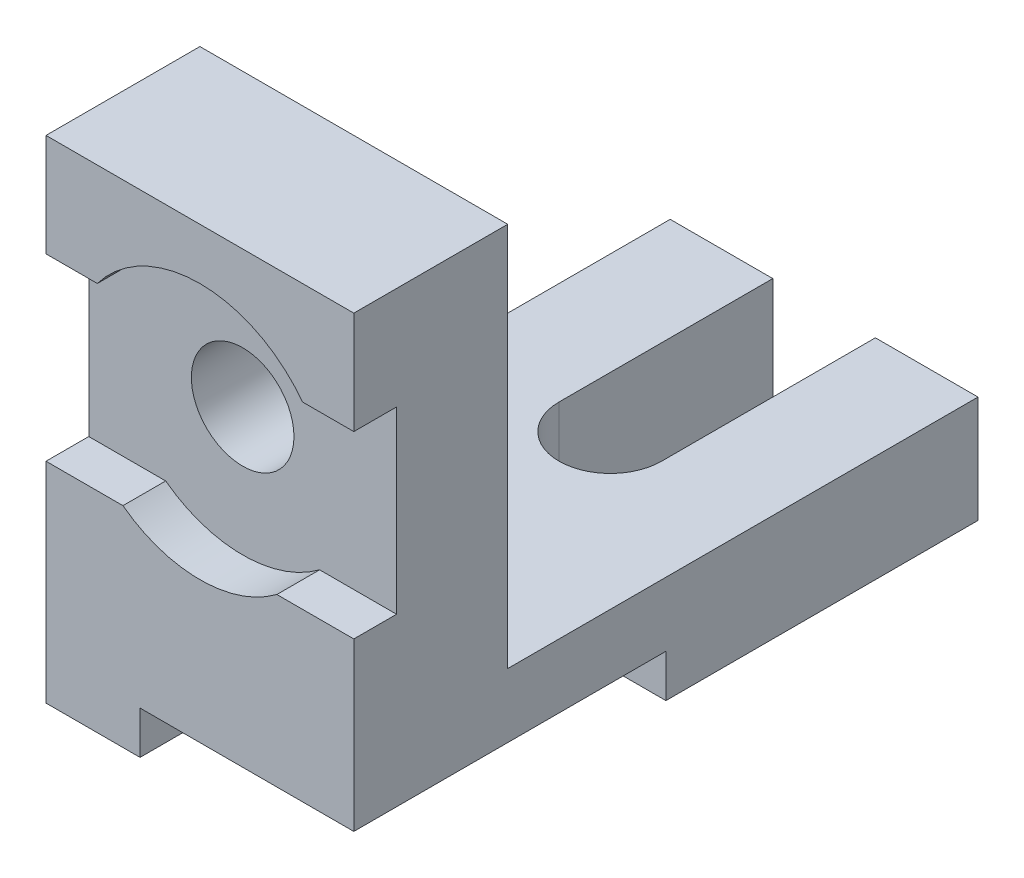
ISO-10303-21;
HEADER;
FILE_DESCRIPTION(('STEP AP214'),'2;1');
FILE_NAME('part.step','',(''),(''),'','','');
FILE_SCHEMA(('AUTOMOTIVE_DESIGN { 1 0 10303 214 1 1 1 1 }'));
ENDSEC;
DATA;
#1=APPLICATION_CONTEXT('core data for automotive mechanical design processes');
#2=APPLICATION_PROTOCOL_DEFINITION('international standard','automotive_design',2000,#1);
#3=PRODUCT_CONTEXT('',#1,'mechanical');
#4=PRODUCT('Part','Part','',(#3));
#5=PRODUCT_RELATED_PRODUCT_CATEGORY('part','',(#4));
#6=PRODUCT_DEFINITION_FORMATION('','',#4);
#7=PRODUCT_DEFINITION_CONTEXT('part definition',#1,'design');
#8=PRODUCT_DEFINITION('design','',#6,#7);
#9=PRODUCT_DEFINITION_SHAPE('','',#8);
#10=(LENGTH_UNIT() NAMED_UNIT(*) SI_UNIT(.MILLI.,.METRE.));
#11=(NAMED_UNIT(*) PLANE_ANGLE_UNIT() SI_UNIT($,.RADIAN.));
#12=(NAMED_UNIT(*) SI_UNIT($,.STERADIAN.) SOLID_ANGLE_UNIT());
#13=UNCERTAINTY_MEASURE_WITH_UNIT(LENGTH_MEASURE(1.E-05),#10,'distance_accuracy_value','');
#14=(GEOMETRIC_REPRESENTATION_CONTEXT(3) GLOBAL_UNCERTAINTY_ASSIGNED_CONTEXT((#13)) GLOBAL_UNIT_ASSIGNED_CONTEXT((#10,
#11,#12)) REPRESENTATION_CONTEXT('',''));
#15=CARTESIAN_POINT('',(0.,0.,0.));
#16=DIRECTION('',(0.,0.,1.));
#17=DIRECTION('',(1.,0.,0.));
#18=AXIS2_PLACEMENT_3D('',#15,#16,#17);
#19=CARTESIAN_POINT('',(-148.124947257375,-25.,-146.));
#20=DIRECTION('',(0.,0.,-1.));
#21=DIRECTION('',(-1.,0.,0.));
#22=AXIS2_PLACEMENT_3D('',#19,#20,#21);
#23=PLANE('',#22);
#24=DIRECTION('',(0.,1.,0.));
#25=VECTOR('',#24,1.);
#26=CARTESIAN_POINT('',(48.,-42.,-146.));
#27=LINE('',#26,#25);
#28=CARTESIAN_POINT('',(48.,-25.,-146.));
#29=VERTEX_POINT('',#28);
#30=CARTESIAN_POINT('',(48.,0.,-146.));
#31=VERTEX_POINT('',#30);
#32=EDGE_CURVE('E216',#29,#31,#27,.T.);
#33=ORIENTED_EDGE('',*,*,#32,.T.);
#34=DIRECTION('',(1.,0.,0.));
#35=VECTOR('',#34,1.);
#36=CARTESIAN_POINT('',(-148.124947257375,0.,-146.));
#37=LINE('',#36,#35);
#38=CARTESIAN_POINT('',(72.,0.,-146.));
#39=VERTEX_POINT('',#38);
#40=EDGE_CURVE('E247',#31,#39,#37,.T.);
#41=ORIENTED_EDGE('',*,*,#40,.T.);
#42=DIRECTION('',(0.,1.,0.));
#43=VECTOR('',#42,1.);
#44=CARTESIAN_POINT('',(72.,-25.,-146.));
#45=LINE('',#44,#43);
#46=CARTESIAN_POINT('',(72.,-25.,-146.));
#47=VERTEX_POINT('',#46);
#48=EDGE_CURVE('E231',#47,#39,#45,.T.);
#49=ORIENTED_EDGE('',*,*,#48,.F.);
#50=DIRECTION('',(1.,0.,0.));
#51=VECTOR('',#50,1.);
#52=CARTESIAN_POINT('',(-148.124947257375,-25.,-146.));
#53=LINE('',#52,#51);
#54=EDGE_CURVE('E252',#29,#47,#53,.T.);
#55=ORIENTED_EDGE('',*,*,#54,.F.);
#56=EDGE_LOOP('',(#33,#41,#49,#55));
#57=FACE_BOUND('',#56,.T.);
#58=ADVANCED_FACE('F39',(#57),#23,.T.);
#59=CARTESIAN_POINT('',(0.,0.,0.));
#60=DIRECTION('',(0.,0.,-1.));
#61=DIRECTION('',(-1.,0.,0.));
#62=AXIS2_PLACEMENT_3D('',#59,#60,#61);
#63=PLANE('',#62);
#64=DIRECTION('',(0.,-1.,0.));
#65=VECTOR('',#64,1.);
#66=CARTESIAN_POINT('',(0.,0.,0.));
#67=LINE('',#66,#65);
#68=CARTESIAN_POINT('',(0.,90.,0.));
#69=VERTEX_POINT('',#68);
#70=CARTESIAN_POINT('',(0.,66.,0.));
#71=VERTEX_POINT('',#70);
#72=EDGE_CURVE('E333',#69,#71,#67,.T.);
#73=ORIENTED_EDGE('',*,*,#72,.T.);
#74=DIRECTION('',(-1.,0.,0.));
#75=VECTOR('',#74,1.);
#76=CARTESIAN_POINT('',(0.,66.,0.));
#77=LINE('',#76,#75);
#78=CARTESIAN_POINT('',(12.,66.,0.));
#79=VERTEX_POINT('',#78);
#80=EDGE_CURVE('E297',#79,#71,#77,.T.);
#81=ORIENTED_EDGE('',*,*,#80,.F.);
#82=CARTESIAN_POINT('',(36.,48.,0.));
#83=DIRECTION('',(0.,0.,1.));
#84=DIRECTION('',(1.,0.,0.));
#85=AXIS2_PLACEMENT_3D('',#82,#83,#84);
#86=CIRCLE('',#85,30.);
#87=CARTESIAN_POINT('',(60.,66.,0.));
#88=VERTEX_POINT('',#87);
#89=EDGE_CURVE('E300',#88,#79,#86,.T.);
#90=ORIENTED_EDGE('',*,*,#89,.F.);
#91=DIRECTION('',(-1.,0.,0.));
#92=VECTOR('',#91,1.);
#93=CARTESIAN_POINT('',(60.,66.,0.));
#94=LINE('',#93,#92);
#95=CARTESIAN_POINT('',(72.,66.,0.));
#96=VERTEX_POINT('',#95);
#97=EDGE_CURVE('E294',#96,#88,#94,.T.);
#98=ORIENTED_EDGE('',*,*,#97,.F.);
#99=DIRECTION('',(0.,1.,0.));
#100=VECTOR('',#99,1.);
#101=CARTESIAN_POINT('',(72.,0.,0.));
#102=LINE('',#101,#100);
#103=CARTESIAN_POINT('',(72.,90.,0.));
#104=VERTEX_POINT('',#103);
#105=EDGE_CURVE('E336',#96,#104,#102,.T.);
#106=ORIENTED_EDGE('',*,*,#105,.T.);
#107=DIRECTION('',(-1.,0.,0.));
#108=VECTOR('',#107,1.);
#109=CARTESIAN_POINT('',(0.,90.,0.));
#110=LINE('',#109,#108);
#111=EDGE_CURVE('E326',#104,#69,#110,.T.);
#112=ORIENTED_EDGE('',*,*,#111,.T.);
#113=EDGE_LOOP('',(#73,#81,#90,#98,#106,#112));
#114=FACE_BOUND('',#113,.T.);
#115=ADVANCED_FACE('F344',(#114),#63,.F.);
#116=CARTESIAN_POINT('',(0.,0.,-36.));
#117=DIRECTION('',(-1.,0.,0.));
#118=DIRECTION('',(0.,0.,1.));
#119=AXIS2_PLACEMENT_3D('',#116,#117,#118);
#120=PLANE('',#119);
#121=DIRECTION('',(0.,0.,1.));
#122=VECTOR('',#121,1.);
#123=CARTESIAN_POINT('',(0.,24.,-10.));
#124=LINE('',#123,#122);
#125=CARTESIAN_POINT('',(0.,24.,-10.));
#126=VERTEX_POINT('',#125);
#127=CARTESIAN_POINT('',(0.,24.,0.));
#128=VERTEX_POINT('',#127);
#129=EDGE_CURVE('E307',#126,#128,#124,.T.);
#130=ORIENTED_EDGE('',*,*,#129,.F.);
#131=DIRECTION('',(0.,-1.,0.));
#132=VECTOR('',#131,1.);
#133=CARTESIAN_POINT('',(0.,66.,-10.));
#134=LINE('',#133,#132);
#135=CARTESIAN_POINT('',(0.,66.,-10.));
#136=VERTEX_POINT('',#135);
#137=EDGE_CURVE('E284',#136,#126,#134,.T.);
#138=ORIENTED_EDGE('',*,*,#137,.F.);
#139=DIRECTION('',(0.,0.,1.));
#140=VECTOR('',#139,1.);
#141=CARTESIAN_POINT('',(0.,66.,-10.));
#142=LINE('',#141,#140);
#143=EDGE_CURVE('E310',#136,#71,#142,.T.);
#144=ORIENTED_EDGE('',*,*,#143,.T.);
#145=ORIENTED_EDGE('',*,*,#72,.F.);
#146=DIRECTION('',(0.,0.,1.));
#147=VECTOR('',#146,1.);
#148=CARTESIAN_POINT('',(0.,90.,-36.));
#149=LINE('',#148,#147);
#150=CARTESIAN_POINT('',(0.,90.,-36.));
#151=VERTEX_POINT('',#150);
#152=EDGE_CURVE('E11',#151,#69,#149,.T.);
#153=ORIENTED_EDGE('',*,*,#152,.F.);
#154=DIRECTION('',(0.,-1.,0.));
#155=VECTOR('',#154,1.);
#156=CARTESIAN_POINT('',(0.,0.,-36.));
#157=LINE('',#156,#155);
#158=CARTESIAN_POINT('',(0.,0.,-36.));
#159=VERTEX_POINT('',#158);
#160=EDGE_CURVE('E325',#151,#159,#157,.T.);
#161=ORIENTED_EDGE('',*,*,#160,.T.);
#162=DIRECTION('',(0.,0.,1.));
#163=VECTOR('',#162,1.);
#164=CARTESIAN_POINT('',(0.,0.,-146.));
#165=LINE('',#164,#163);
#166=CARTESIAN_POINT('',(0.,0.,-146.));
#167=VERTEX_POINT('',#166);
#168=EDGE_CURVE('E239',#167,#159,#165,.T.);
#169=ORIENTED_EDGE('',*,*,#168,.F.);
#170=DIRECTION('',(0.,1.,0.));
#171=VECTOR('',#170,1.);
#172=CARTESIAN_POINT('',(0.,-25.,-146.));
#173=LINE('',#172,#171);
#174=CARTESIAN_POINT('',(0.,-25.,-146.));
#175=VERTEX_POINT('',#174);
#176=EDGE_CURVE('E244',#175,#167,#173,.T.);
#177=ORIENTED_EDGE('',*,*,#176,.F.);
#178=DIRECTION('',(0.,0.,-1.));
#179=VECTOR('',#178,1.);
#180=CARTESIAN_POINT('',(0.,-25.,0.));
#181=LINE('',#180,#179);
#182=CARTESIAN_POINT('',(0.,-25.,0.));
#183=VERTEX_POINT('',#182);
#184=EDGE_CURVE('E248',#183,#175,#181,.T.);
#185=ORIENTED_EDGE('',*,*,#184,.F.);
#186=EDGE_CURVE('E308',#128,#183,#67,.T.);
#187=ORIENTED_EDGE('',*,*,#186,.F.);
#188=EDGE_LOOP('',(#130,#138,#144,#145,#153,#161,#169,#177,#185,#187));
#189=FACE_BOUND('',#188,.T.);
#190=ADVANCED_FACE('F41',(#189),#120,.T.);
#191=CARTESIAN_POINT('',(0.,90.,-36.));
#192=DIRECTION('',(0.,1.,0.));
#193=DIRECTION('',(0.,0.,1.));
#194=AXIS2_PLACEMENT_3D('',#191,#192,#193);
#195=PLANE('',#194);
#196=ORIENTED_EDGE('',*,*,#111,.F.);
#197=DIRECTION('',(0.,0.,1.));
#198=VECTOR('',#197,1.);
#199=CARTESIAN_POINT('',(72.,90.,-36.));
#200=LINE('',#199,#198);
#201=CARTESIAN_POINT('',(72.,90.,-36.));
#202=VERTEX_POINT('',#201);
#203=EDGE_CURVE('E43',#202,#104,#200,.T.);
#204=ORIENTED_EDGE('',*,*,#203,.F.);
#205=DIRECTION('',(-1.,0.,0.));
#206=VECTOR('',#205,1.);
#207=CARTESIAN_POINT('',(0.,90.,-36.));
#208=LINE('',#207,#206);
#209=EDGE_CURVE('E335',#202,#151,#208,.T.);
#210=ORIENTED_EDGE('',*,*,#209,.T.);
#211=ORIENTED_EDGE('',*,*,#152,.T.);
#212=EDGE_LOOP('',(#196,#204,#210,#211));
#213=FACE_BOUND('',#212,.T.);
#214=ADVANCED_FACE('F348',(#213),#195,.T.);
#215=CARTESIAN_POINT('',(72.,0.,-36.));
#216=DIRECTION('',(1.,0.,0.));
#217=DIRECTION('',(0.,0.,-1.));
#218=AXIS2_PLACEMENT_3D('',#215,#216,#217);
#219=PLANE('',#218);
#220=DIRECTION('',(0.,0.,1.));
#221=VECTOR('',#220,1.);
#222=CARTESIAN_POINT('',(72.,-15.,-73.));
#223=LINE('',#222,#221);
#224=CARTESIAN_POINT('',(72.,-15.,-73.));
#225=VERTEX_POINT('',#224);
#226=CARTESIAN_POINT('',(72.,-15.,0.));
#227=VERTEX_POINT('',#226);
#228=EDGE_CURVE('E188',#225,#227,#223,.T.);
#229=ORIENTED_EDGE('',*,*,#228,.F.);
#230=DIRECTION('',(0.,1.,0.));
#231=VECTOR('',#230,1.);
#232=CARTESIAN_POINT('',(72.,-25.,-73.));
#233=LINE('',#232,#231);
#234=CARTESIAN_POINT('',(72.,-25.,-73.));
#235=VERTEX_POINT('',#234);
#236=EDGE_CURVE('E189',#235,#225,#233,.T.);
#237=ORIENTED_EDGE('',*,*,#236,.F.);
#238=DIRECTION('',(0.,0.,-1.));
#239=VECTOR('',#238,1.);
#240=CARTESIAN_POINT('',(72.,-25.,0.));
#241=LINE('',#240,#239);
#242=EDGE_CURVE('E235',#235,#47,#241,.T.);
#243=ORIENTED_EDGE('',*,*,#242,.T.);
#244=ORIENTED_EDGE('',*,*,#48,.T.);
#245=DIRECTION('',(0.,0.,1.));
#246=VECTOR('',#245,1.);
#247=CARTESIAN_POINT('',(72.,0.,-146.));
#248=LINE('',#247,#246);
#249=CARTESIAN_POINT('',(72.,0.,-36.));
#250=VERTEX_POINT('',#249);
#251=EDGE_CURVE('E227',#39,#250,#248,.T.);
#252=ORIENTED_EDGE('',*,*,#251,.T.);
#253=DIRECTION('',(0.,1.,0.));
#254=VECTOR('',#253,1.);
#255=CARTESIAN_POINT('',(72.,0.,-36.));
#256=LINE('',#255,#254);
#257=EDGE_CURVE('E328',#250,#202,#256,.T.);
#258=ORIENTED_EDGE('',*,*,#257,.T.);
#259=ORIENTED_EDGE('',*,*,#203,.T.);
#260=ORIENTED_EDGE('',*,*,#105,.F.);
#261=DIRECTION('',(0.,0.,1.));
#262=VECTOR('',#261,1.);
#263=CARTESIAN_POINT('',(72.,66.,-10.));
#264=LINE('',#263,#262);
#265=CARTESIAN_POINT('',(72.,66.,-10.));
#266=VERTEX_POINT('',#265);
#267=EDGE_CURVE('E316',#266,#96,#264,.T.);
#268=ORIENTED_EDGE('',*,*,#267,.F.);
#269=DIRECTION('',(0.,1.,0.));
#270=VECTOR('',#269,1.);
#271=CARTESIAN_POINT('',(72.,24.,-10.));
#272=LINE('',#271,#270);
#273=CARTESIAN_POINT('',(72.,24.,-10.));
#274=VERTEX_POINT('',#273);
#275=EDGE_CURVE('E275',#274,#266,#272,.T.);
#276=ORIENTED_EDGE('',*,*,#275,.F.);
#277=DIRECTION('',(0.,0.,1.));
#278=VECTOR('',#277,1.);
#279=CARTESIAN_POINT('',(72.,24.,-10.));
#280=LINE('',#279,#278);
#281=CARTESIAN_POINT('',(72.,24.,0.));
#282=VERTEX_POINT('',#281);
#283=EDGE_CURVE('E318',#274,#282,#280,.T.);
#284=ORIENTED_EDGE('',*,*,#283,.T.);
#285=EDGE_CURVE('E205',#227,#282,#102,.T.);
#286=ORIENTED_EDGE('',*,*,#285,.F.);
#287=EDGE_LOOP('',(#229,#237,#243,#244,#252,#258,#259,#260,#268,#276,#284,#286));
#288=FACE_BOUND('',#287,.T.);
#289=ADVANCED_FACE('F199',(#288),#219,.T.);
#290=CARTESIAN_POINT('',(0.,0.,-36.));
#291=DIRECTION('',(0.,0.,-1.));
#292=DIRECTION('',(-1.,0.,0.));
#293=AXIS2_PLACEMENT_3D('',#290,#291,#292);
#294=PLANE('',#293);
#295=CARTESIAN_POINT('',(36.,48.,-36.));
#296=DIRECTION('',(0.,0.,-1.));
#297=DIRECTION('',(-1.,0.,0.));
#298=AXIS2_PLACEMENT_3D('',#295,#296,#297);
#299=CIRCLE('',#298,12.);
#300=CARTESIAN_POINT('',(24.,48.,-36.));
#301=VERTEX_POINT('',#300);
#302=EDGE_CURVE('E261',#301,#301,#299,.T.);
#303=ORIENTED_EDGE('',*,*,#302,.F.);
#304=EDGE_LOOP('',(#303));
#305=FACE_BOUND('',#304,.T.);
#306=ORIENTED_EDGE('',*,*,#160,.F.);
#307=ORIENTED_EDGE('',*,*,#209,.F.);
#308=ORIENTED_EDGE('',*,*,#257,.F.);
#309=DIRECTION('',(1.,0.,0.));
#310=VECTOR('',#309,1.);
#311=CARTESIAN_POINT('',(0.,0.,-36.));
#312=LINE('',#311,#310);
#313=EDGE_CURVE('E324',#159,#250,#312,.T.);
#314=ORIENTED_EDGE('',*,*,#313,.F.);
#315=EDGE_LOOP('',(#306,#307,#308,#314));
#316=FACE_BOUND('',#315,.T.);
#317=ADVANCED_FACE('F371',(#305,#316),#294,.T.);
#318=DIRECTION('',(1.,0.,0.));
#319=VECTOR('',#318,1.);
#320=CARTESIAN_POINT('',(-148.124947257375,-25.,0.));
#321=LINE('',#320,#319);
#322=CARTESIAN_POINT('',(22.,-25.,0.));
#323=VERTEX_POINT('',#322);
#324=EDGE_CURVE('E233',#183,#323,#321,.T.);
#325=ORIENTED_EDGE('',*,*,#324,.T.);
#326=DIRECTION('',(0.,-1.,0.));
#327=VECTOR('',#326,1.);
#328=CARTESIAN_POINT('',(22.,-25.,0.));
#329=LINE('',#328,#327);
#330=CARTESIAN_POINT('',(22.,-15.,0.));
#331=VERTEX_POINT('',#330);
#332=EDGE_CURVE('E197',#331,#323,#329,.T.);
#333=ORIENTED_EDGE('',*,*,#332,.F.);
#334=DIRECTION('',(-1.,0.,0.));
#335=VECTOR('',#334,1.);
#336=CARTESIAN_POINT('',(72.,-15.,0.));
#337=LINE('',#336,#335);
#338=EDGE_CURVE('E400',#227,#331,#337,.T.);
#339=ORIENTED_EDGE('',*,*,#338,.F.);
#340=ORIENTED_EDGE('',*,*,#285,.T.);
#341=DIRECTION('',(1.,0.,0.));
#342=VECTOR('',#341,1.);
#343=CARTESIAN_POINT('',(54.,24.,0.));
#344=LINE('',#343,#342);
#345=CARTESIAN_POINT('',(54.,24.,0.));
#346=VERTEX_POINT('',#345);
#347=EDGE_CURVE('E292',#346,#282,#344,.T.);
#348=ORIENTED_EDGE('',*,*,#347,.F.);
#349=CARTESIAN_POINT('',(36.,48.,0.));
#350=DIRECTION('',(0.,0.,1.));
#351=DIRECTION('',(1.,0.,0.));
#352=AXIS2_PLACEMENT_3D('',#349,#350,#351);
#353=CIRCLE('',#352,30.);
#354=CARTESIAN_POINT('',(18.,24.,0.));
#355=VERTEX_POINT('',#354);
#356=EDGE_CURVE('E262',#355,#346,#353,.T.);
#357=ORIENTED_EDGE('',*,*,#356,.F.);
#358=DIRECTION('',(1.,0.,0.));
#359=VECTOR('',#358,1.);
#360=CARTESIAN_POINT('',(0.,24.,0.));
#361=LINE('',#360,#359);
#362=EDGE_CURVE('E267',#128,#355,#361,.T.);
#363=ORIENTED_EDGE('',*,*,#362,.F.);
#364=ORIENTED_EDGE('',*,*,#186,.T.);
#365=EDGE_LOOP('',(#325,#333,#339,#340,#348,#357,#363,#364));
#366=FACE_BOUND('',#365,.T.);
#367=ADVANCED_FACE('F389',(#366),#63,.F.);
#368=CARTESIAN_POINT('',(36.,48.,-10.));
#369=DIRECTION('',(0.,0.,1.));
#370=DIRECTION('',(1.,0.,0.));
#371=AXIS2_PLACEMENT_3D('',#368,#369,#370);
#372=CYLINDRICAL_SURFACE('',#371,30.);
#373=ORIENTED_EDGE('',*,*,#356,.T.);
#374=DIRECTION('',(0.,0.,1.));
#375=VECTOR('',#374,1.);
#376=CARTESIAN_POINT('',(54.,24.,-10.));
#377=LINE('',#376,#375);
#378=CARTESIAN_POINT('',(54.,24.,-10.));
#379=VERTEX_POINT('',#378);
#380=EDGE_CURVE('E288',#379,#346,#377,.T.);
#381=ORIENTED_EDGE('',*,*,#380,.F.);
#382=CARTESIAN_POINT('',(36.,48.,-10.));
#383=DIRECTION('',(0.,0.,1.));
#384=DIRECTION('',(1.,0.,0.));
#385=AXIS2_PLACEMENT_3D('',#382,#383,#384);
#386=CIRCLE('',#385,30.);
#387=CARTESIAN_POINT('',(18.,24.,-10.));
#388=VERTEX_POINT('',#387);
#389=EDGE_CURVE('E264',#388,#379,#386,.T.);
#390=ORIENTED_EDGE('',*,*,#389,.F.);
#391=DIRECTION('',(0.,0.,1.));
#392=VECTOR('',#391,1.);
#393=CARTESIAN_POINT('',(18.,24.,-10.));
#394=LINE('',#393,#392);
#395=EDGE_CURVE('E303',#388,#355,#394,.T.);
#396=ORIENTED_EDGE('',*,*,#395,.T.);
#397=EDGE_LOOP('',(#373,#381,#390,#396));
#398=FACE_BOUND('',#397,.T.);
#399=ADVANCED_FACE('F397',(#398),#372,.F.);
#400=CARTESIAN_POINT('',(0.,24.,-10.));
#401=DIRECTION('',(0.,-1.,0.));
#402=DIRECTION('',(0.,0.,-1.));
#403=AXIS2_PLACEMENT_3D('',#400,#401,#402);
#404=PLANE('',#403);
#405=ORIENTED_EDGE('',*,*,#362,.T.);
#406=ORIENTED_EDGE('',*,*,#395,.F.);
#407=DIRECTION('',(1.,0.,0.));
#408=VECTOR('',#407,1.);
#409=CARTESIAN_POINT('',(0.,24.,-10.));
#410=LINE('',#409,#408);
#411=EDGE_CURVE('E286',#126,#388,#410,.T.);
#412=ORIENTED_EDGE('',*,*,#411,.F.);
#413=ORIENTED_EDGE('',*,*,#129,.T.);
#414=EDGE_LOOP('',(#405,#406,#412,#413));
#415=FACE_BOUND('',#414,.T.);
#416=ADVANCED_FACE('F391',(#415),#404,.F.);
#417=CARTESIAN_POINT('',(0.,66.,-10.));
#418=DIRECTION('',(0.,1.,0.));
#419=DIRECTION('',(0.,0.,1.));
#420=AXIS2_PLACEMENT_3D('',#417,#418,#419);
#421=PLANE('',#420);
#422=ORIENTED_EDGE('',*,*,#80,.T.);
#423=ORIENTED_EDGE('',*,*,#143,.F.);
#424=DIRECTION('',(-1.,0.,0.));
#425=VECTOR('',#424,1.);
#426=CARTESIAN_POINT('',(0.,66.,-10.));
#427=LINE('',#426,#425);
#428=CARTESIAN_POINT('',(12.,66.,-10.));
#429=VERTEX_POINT('',#428);
#430=EDGE_CURVE('E283',#429,#136,#427,.T.);
#431=ORIENTED_EDGE('',*,*,#430,.F.);
#432=DIRECTION('',(0.,0.,1.));
#433=VECTOR('',#432,1.);
#434=CARTESIAN_POINT('',(12.,66.,-10.));
#435=LINE('',#434,#433);
#436=EDGE_CURVE('E315',#429,#79,#435,.T.);
#437=ORIENTED_EDGE('',*,*,#436,.T.);
#438=EDGE_LOOP('',(#422,#423,#431,#437));
#439=FACE_BOUND('',#438,.T.);
#440=ADVANCED_FACE('F359',(#439),#421,.F.);
#441=CARTESIAN_POINT('',(36.,48.,-10.));
#442=DIRECTION('',(0.,0.,1.));
#443=DIRECTION('',(1.,0.,0.));
#444=AXIS2_PLACEMENT_3D('',#441,#442,#443);
#445=CYLINDRICAL_SURFACE('',#444,30.);
#446=ORIENTED_EDGE('',*,*,#89,.T.);
#447=ORIENTED_EDGE('',*,*,#436,.F.);
#448=CARTESIAN_POINT('',(36.,48.,-10.));
#449=DIRECTION('',(0.,0.,1.));
#450=DIRECTION('',(1.,0.,0.));
#451=AXIS2_PLACEMENT_3D('',#448,#449,#450);
#452=CIRCLE('',#451,30.);
#453=CARTESIAN_POINT('',(60.,66.,-10.));
#454=VERTEX_POINT('',#453);
#455=EDGE_CURVE('E279',#454,#429,#452,.T.);
#456=ORIENTED_EDGE('',*,*,#455,.F.);
#457=DIRECTION('',(0.,0.,1.));
#458=VECTOR('',#457,1.);
#459=CARTESIAN_POINT('',(60.,66.,-10.));
#460=LINE('',#459,#458);
#461=EDGE_CURVE('E314',#454,#88,#460,.T.);
#462=ORIENTED_EDGE('',*,*,#461,.T.);
#463=EDGE_LOOP('',(#446,#447,#456,#462));
#464=FACE_BOUND('',#463,.T.);
#465=ADVANCED_FACE('F365',(#464),#445,.F.);
#466=CARTESIAN_POINT('',(60.,66.,-10.));
#467=DIRECTION('',(0.,1.,0.));
#468=DIRECTION('',(0.,0.,1.));
#469=AXIS2_PLACEMENT_3D('',#466,#467,#468);
#470=PLANE('',#469);
#471=ORIENTED_EDGE('',*,*,#97,.T.);
#472=ORIENTED_EDGE('',*,*,#461,.F.);
#473=DIRECTION('',(-1.,0.,0.));
#474=VECTOR('',#473,1.);
#475=CARTESIAN_POINT('',(60.,66.,-10.));
#476=LINE('',#475,#474);
#477=EDGE_CURVE('E274',#266,#454,#476,.T.);
#478=ORIENTED_EDGE('',*,*,#477,.F.);
#479=ORIENTED_EDGE('',*,*,#267,.T.);
#480=EDGE_LOOP('',(#471,#472,#478,#479));
#481=FACE_BOUND('',#480,.T.);
#482=ADVANCED_FACE('F463',(#481),#470,.F.);
#483=CARTESIAN_POINT('',(54.,24.,-10.));
#484=DIRECTION('',(0.,-1.,0.));
#485=DIRECTION('',(0.,0.,-1.));
#486=AXIS2_PLACEMENT_3D('',#483,#484,#485);
#487=PLANE('',#486);
#488=ORIENTED_EDGE('',*,*,#347,.T.);
#489=ORIENTED_EDGE('',*,*,#283,.F.);
#490=DIRECTION('',(1.,0.,0.));
#491=VECTOR('',#490,1.);
#492=CARTESIAN_POINT('',(54.,24.,-10.));
#493=LINE('',#492,#491);
#494=EDGE_CURVE('E268',#379,#274,#493,.T.);
#495=ORIENTED_EDGE('',*,*,#494,.F.);
#496=ORIENTED_EDGE('',*,*,#380,.T.);
#497=EDGE_LOOP('',(#488,#489,#495,#496));
#498=FACE_BOUND('',#497,.T.);
#499=ADVANCED_FACE('F398',(#498),#487,.F.);
#500=CARTESIAN_POINT('',(36.,48.,-10.));
#501=DIRECTION('',(0.,0.,1.));
#502=DIRECTION('',(1.,0.,0.));
#503=AXIS2_PLACEMENT_3D('',#500,#501,#502);
#504=PLANE('',#503);
#505=CARTESIAN_POINT('',(36.,48.,-10.));
#506=DIRECTION('',(0.,0.,1.));
#507=DIRECTION('',(1.,0.,0.));
#508=AXIS2_PLACEMENT_3D('',#505,#506,#507);
#509=CIRCLE('',#508,12.);
#510=CARTESIAN_POINT('',(48.,48.,-10.));
#511=VERTEX_POINT('',#510);
#512=EDGE_CURVE('E245',#511,#511,#509,.T.);
#513=ORIENTED_EDGE('',*,*,#512,.F.);
#514=EDGE_LOOP('',(#513));
#515=FACE_BOUND('',#514,.T.);
#516=ORIENTED_EDGE('',*,*,#389,.T.);
#517=ORIENTED_EDGE('',*,*,#494,.T.);
#518=ORIENTED_EDGE('',*,*,#275,.T.);
#519=ORIENTED_EDGE('',*,*,#477,.T.);
#520=ORIENTED_EDGE('',*,*,#455,.T.);
#521=ORIENTED_EDGE('',*,*,#430,.T.);
#522=ORIENTED_EDGE('',*,*,#137,.T.);
#523=ORIENTED_EDGE('',*,*,#411,.T.);
#524=EDGE_LOOP('',(#516,#517,#518,#519,#520,#521,#522,#523));
#525=FACE_BOUND('',#524,.T.);
#526=ADVANCED_FACE('F360',(#515,#525),#504,.T.);
#527=CARTESIAN_POINT('',(36.,48.,-52.));
#528=DIRECTION('',(0.,0.,1.));
#529=DIRECTION('',(1.,0.,0.));
#530=AXIS2_PLACEMENT_3D('',#527,#528,#529);
#531=CYLINDRICAL_SURFACE('',#530,12.);
#532=ORIENTED_EDGE('',*,*,#302,.T.);
#533=EDGE_LOOP('',(#532));
#534=FACE_BOUND('',#533,.T.);
#535=ORIENTED_EDGE('',*,*,#512,.T.);
#536=EDGE_LOOP('',(#535));
#537=FACE_BOUND('',#536,.T.);
#538=ADVANCED_FACE('F441',(#534,#537),#531,.F.);
#539=CARTESIAN_POINT('',(-148.124947257375,-25.,0.));
#540=DIRECTION('',(0.,-1.,0.));
#541=DIRECTION('',(0.,0.,-1.));
#542=AXIS2_PLACEMENT_3D('',#539,#540,#541);
#543=PLANE('',#542);
#544=DIRECTION('',(0.,0.,1.));
#545=VECTOR('',#544,1.);
#546=CARTESIAN_POINT('',(22.,-25.,-73.));
#547=LINE('',#546,#545);
#548=CARTESIAN_POINT('',(22.,-25.,-73.));
#549=VERTEX_POINT('',#548);
#550=EDGE_CURVE('E204',#549,#323,#547,.T.);
#551=ORIENTED_EDGE('',*,*,#550,.T.);
#552=ORIENTED_EDGE('',*,*,#324,.F.);
#553=ORIENTED_EDGE('',*,*,#184,.T.);
#554=CARTESIAN_POINT('',(24.,-25.,-146.));
#555=VERTEX_POINT('',#554);
#556=EDGE_CURVE('E249',#175,#555,#53,.T.);
#557=ORIENTED_EDGE('',*,*,#556,.T.);
#558=DIRECTION('',(0.,0.,-1.));
#559=VECTOR('',#558,1.);
#560=CARTESIAN_POINT('',(24.,-25.,0.));
#561=LINE('',#560,#559);
#562=CARTESIAN_POINT('',(24.,-25.,-96.));
#563=VERTEX_POINT('',#562);
#564=EDGE_CURVE('E218',#563,#555,#561,.T.);
#565=ORIENTED_EDGE('',*,*,#564,.F.);
#566=CARTESIAN_POINT('',(36.,-25.,-96.));
#567=DIRECTION('',(0.,-1.,0.));
#568=DIRECTION('',(0.,0.,-1.));
#569=AXIS2_PLACEMENT_3D('',#566,#567,#568);
#570=CIRCLE('',#569,12.);
#571=CARTESIAN_POINT('',(48.,-25.,-96.));
#572=VERTEX_POINT('',#571);
#573=EDGE_CURVE('E228',#572,#563,#570,.T.);
#574=ORIENTED_EDGE('',*,*,#573,.F.);
#575=DIRECTION('',(0.,0.,1.));
#576=VECTOR('',#575,1.);
#577=CARTESIAN_POINT('',(48.,-25.,0.));
#578=LINE('',#577,#576);
#579=EDGE_CURVE('E226',#29,#572,#578,.T.);
#580=ORIENTED_EDGE('',*,*,#579,.F.);
#581=ORIENTED_EDGE('',*,*,#54,.T.);
#582=ORIENTED_EDGE('',*,*,#242,.F.);
#583=DIRECTION('',(1.,0.,0.));
#584=VECTOR('',#583,1.);
#585=CARTESIAN_POINT('',(72.,-25.,-73.));
#586=LINE('',#585,#584);
#587=EDGE_CURVE('E193',#549,#235,#586,.T.);
#588=ORIENTED_EDGE('',*,*,#587,.F.);
#589=EDGE_LOOP('',(#551,#552,#553,#557,#565,#574,#580,#581,#582,#588));
#590=FACE_BOUND('',#589,.T.);
#591=ADVANCED_FACE('F384',(#590),#543,.T.);
#592=DIRECTION('',(0.,1.,0.));
#593=VECTOR('',#592,1.);
#594=CARTESIAN_POINT('',(24.,-42.,-146.));
#595=LINE('',#594,#593);
#596=CARTESIAN_POINT('',(24.,0.,-146.));
#597=VERTEX_POINT('',#596);
#598=EDGE_CURVE('E65',#555,#597,#595,.T.);
#599=ORIENTED_EDGE('',*,*,#598,.F.);
#600=ORIENTED_EDGE('',*,*,#556,.F.);
#601=ORIENTED_EDGE('',*,*,#176,.T.);
#602=EDGE_CURVE('E241',#167,#597,#37,.T.);
#603=ORIENTED_EDGE('',*,*,#602,.T.);
#604=EDGE_LOOP('',(#599,#600,#601,#603));
#605=FACE_BOUND('',#604,.T.);
#606=ADVANCED_FACE('F377',(#605),#23,.T.);
#607=CARTESIAN_POINT('',(-148.124947257375,0.,-146.));
#608=DIRECTION('',(0.,1.,0.));
#609=DIRECTION('',(0.,0.,1.));
#610=AXIS2_PLACEMENT_3D('',#607,#608,#609);
#611=PLANE('',#610);
#612=DIRECTION('',(0.,0.,-1.));
#613=VECTOR('',#612,1.);
#614=CARTESIAN_POINT('',(48.,0.,-96.));
#615=LINE('',#614,#613);
#616=CARTESIAN_POINT('',(48.,0.,-96.));
#617=VERTEX_POINT('',#616);
#618=EDGE_CURVE('E212',#617,#31,#615,.T.);
#619=ORIENTED_EDGE('',*,*,#618,.F.);
#620=CARTESIAN_POINT('',(36.,0.,-96.));
#621=DIRECTION('',(0.,1.,0.));
#622=DIRECTION('',(0.,0.,1.));
#623=AXIS2_PLACEMENT_3D('',#620,#621,#622);
#624=CIRCLE('',#623,12.);
#625=CARTESIAN_POINT('',(24.,0.,-96.));
#626=VERTEX_POINT('',#625);
#627=EDGE_CURVE('E211',#626,#617,#624,.T.);
#628=ORIENTED_EDGE('',*,*,#627,.F.);
#629=DIRECTION('',(0.,0.,1.));
#630=VECTOR('',#629,1.);
#631=CARTESIAN_POINT('',(24.,0.,-146.));
#632=LINE('',#631,#630);
#633=EDGE_CURVE('E207',#597,#626,#632,.T.);
#634=ORIENTED_EDGE('',*,*,#633,.F.);
#635=ORIENTED_EDGE('',*,*,#602,.F.);
#636=ORIENTED_EDGE('',*,*,#168,.T.);
#637=ORIENTED_EDGE('',*,*,#313,.T.);
#638=ORIENTED_EDGE('',*,*,#251,.F.);
#639=ORIENTED_EDGE('',*,*,#40,.F.);
#640=EDGE_LOOP('',(#619,#628,#634,#635,#636,#637,#638,#639));
#641=FACE_BOUND('',#640,.T.);
#642=ADVANCED_FACE('F374',(#641),#611,.T.);
#643=CARTESIAN_POINT('',(48.,-42.,-96.));
#644=DIRECTION('',(1.,0.,0.));
#645=DIRECTION('',(0.,0.,-1.));
#646=AXIS2_PLACEMENT_3D('',#643,#644,#645);
#647=PLANE('',#646);
#648=ORIENTED_EDGE('',*,*,#579,.T.);
#649=DIRECTION('',(0.,1.,0.));
#650=VECTOR('',#649,1.);
#651=CARTESIAN_POINT('',(48.,-42.,-96.));
#652=LINE('',#651,#650);
#653=EDGE_CURVE('E219',#572,#617,#652,.T.);
#654=ORIENTED_EDGE('',*,*,#653,.T.);
#655=ORIENTED_EDGE('',*,*,#618,.T.);
#656=ORIENTED_EDGE('',*,*,#32,.F.);
#657=EDGE_LOOP('',(#648,#654,#655,#656));
#658=FACE_BOUND('',#657,.T.);
#659=ADVANCED_FACE('F414',(#658),#647,.F.);
#660=CARTESIAN_POINT('',(36.,-42.,-96.));
#661=DIRECTION('',(0.,1.,0.));
#662=DIRECTION('',(0.,0.,1.));
#663=AXIS2_PLACEMENT_3D('',#660,#661,#662);
#664=CYLINDRICAL_SURFACE('',#663,12.);
#665=ORIENTED_EDGE('',*,*,#573,.T.);
#666=DIRECTION('',(0.,1.,0.));
#667=VECTOR('',#666,1.);
#668=CARTESIAN_POINT('',(24.,-42.,-96.));
#669=LINE('',#668,#667);
#670=EDGE_CURVE('E225',#563,#626,#669,.T.);
#671=ORIENTED_EDGE('',*,*,#670,.T.);
#672=ORIENTED_EDGE('',*,*,#627,.T.);
#673=ORIENTED_EDGE('',*,*,#653,.F.);
#674=EDGE_LOOP('',(#665,#671,#672,#673));
#675=FACE_BOUND('',#674,.T.);
#676=ADVANCED_FACE('F417',(#675),#664,.F.);
#677=CARTESIAN_POINT('',(24.,-42.,-146.));
#678=DIRECTION('',(-1.,0.,0.));
#679=DIRECTION('',(0.,0.,1.));
#680=AXIS2_PLACEMENT_3D('',#677,#678,#679);
#681=PLANE('',#680);
#682=ORIENTED_EDGE('',*,*,#564,.T.);
#683=ORIENTED_EDGE('',*,*,#598,.T.);
#684=ORIENTED_EDGE('',*,*,#633,.T.);
#685=ORIENTED_EDGE('',*,*,#670,.F.);
#686=EDGE_LOOP('',(#682,#683,#684,#685));
#687=FACE_BOUND('',#686,.T.);
#688=ADVANCED_FACE('F419',(#687),#681,.F.);
#689=CARTESIAN_POINT('',(22.,-25.,-73.));
#690=DIRECTION('',(-1.,0.,0.));
#691=DIRECTION('',(0.,0.,1.));
#692=AXIS2_PLACEMENT_3D('',#689,#690,#691);
#693=PLANE('',#692);
#694=ORIENTED_EDGE('',*,*,#332,.T.);
#695=ORIENTED_EDGE('',*,*,#550,.F.);
#696=DIRECTION('',(0.,-1.,0.));
#697=VECTOR('',#696,1.);
#698=CARTESIAN_POINT('',(22.,-25.,-73.));
#699=LINE('',#698,#697);
#700=CARTESIAN_POINT('',(22.,-15.,-73.));
#701=VERTEX_POINT('',#700);
#702=EDGE_CURVE('E53',#701,#549,#699,.T.);
#703=ORIENTED_EDGE('',*,*,#702,.F.);
#704=DIRECTION('',(0.,0.,1.));
#705=VECTOR('',#704,1.);
#706=CARTESIAN_POINT('',(22.,-15.,-73.));
#707=LINE('',#706,#705);
#708=EDGE_CURVE('E186',#701,#331,#707,.T.);
#709=ORIENTED_EDGE('',*,*,#708,.T.);
#710=EDGE_LOOP('',(#694,#695,#703,#709));
#711=FACE_BOUND('',#710,.T.);
#712=ADVANCED_FACE('F403',(#711),#693,.F.);
#713=CARTESIAN_POINT('',(72.,-15.,-73.));
#714=DIRECTION('',(0.,1.,0.));
#715=DIRECTION('',(-1.,0.,0.));
#716=AXIS2_PLACEMENT_3D('',#713,#714,#715);
#717=PLANE('',#716);
#718=ORIENTED_EDGE('',*,*,#338,.T.);
#719=ORIENTED_EDGE('',*,*,#708,.F.);
#720=DIRECTION('',(-1.,0.,0.));
#721=VECTOR('',#720,1.);
#722=CARTESIAN_POINT('',(72.,-15.,-73.));
#723=LINE('',#722,#721);
#724=EDGE_CURVE('E182',#225,#701,#723,.T.);
#725=ORIENTED_EDGE('',*,*,#724,.F.);
#726=ORIENTED_EDGE('',*,*,#228,.T.);
#727=EDGE_LOOP('',(#718,#719,#725,#726));
#728=FACE_BOUND('',#727,.T.);
#729=ADVANCED_FACE('F184',(#728),#717,.F.);
#730=CARTESIAN_POINT('',(0.,0.,-73.));
#731=DIRECTION('',(0.,0.,1.));
#732=DIRECTION('',(1.,0.,0.));
#733=AXIS2_PLACEMENT_3D('',#730,#731,#732);
#734=PLANE('',#733);
#735=ORIENTED_EDGE('',*,*,#236,.T.);
#736=ORIENTED_EDGE('',*,*,#724,.T.);
#737=ORIENTED_EDGE('',*,*,#702,.T.);
#738=ORIENTED_EDGE('',*,*,#587,.T.);
#739=EDGE_LOOP('',(#735,#736,#737,#738));
#740=FACE_BOUND('',#739,.T.);
#741=ADVANCED_FACE('F192',(#740),#734,.T.);
#742=CLOSED_SHELL('',(#58,#115,#190,#214,#289,#317,#367,#399,#416,#440,#465,#482,#499,#526,#538,
#591,#606,#642,#659,#676,#688,#712,#729,#741));
#743=MANIFOLD_SOLID_BREP('B2',#742);
#744=ADVANCED_BREP_SHAPE_REPRESENTATION('',(#18,#743),#14);
#745=SHAPE_DEFINITION_REPRESENTATION(#9,#744);
ENDSEC;
END-ISO-10303-21;
